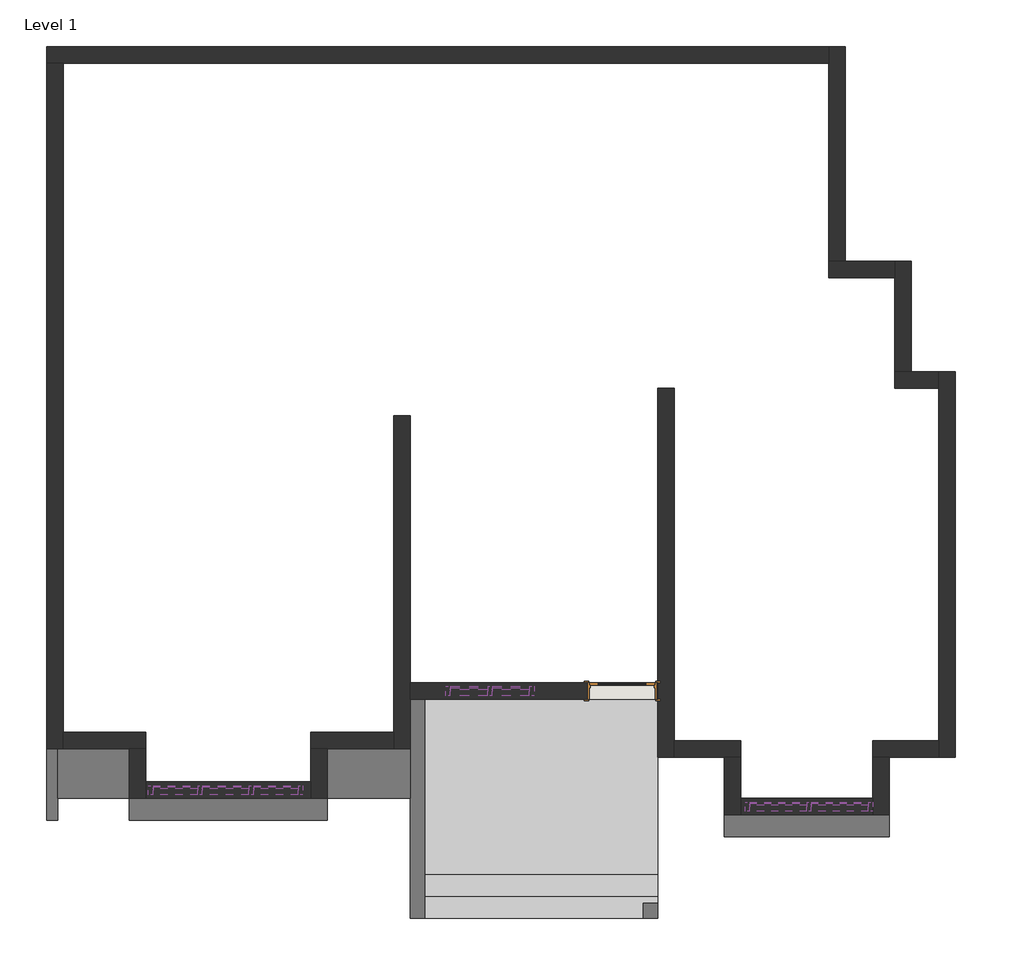
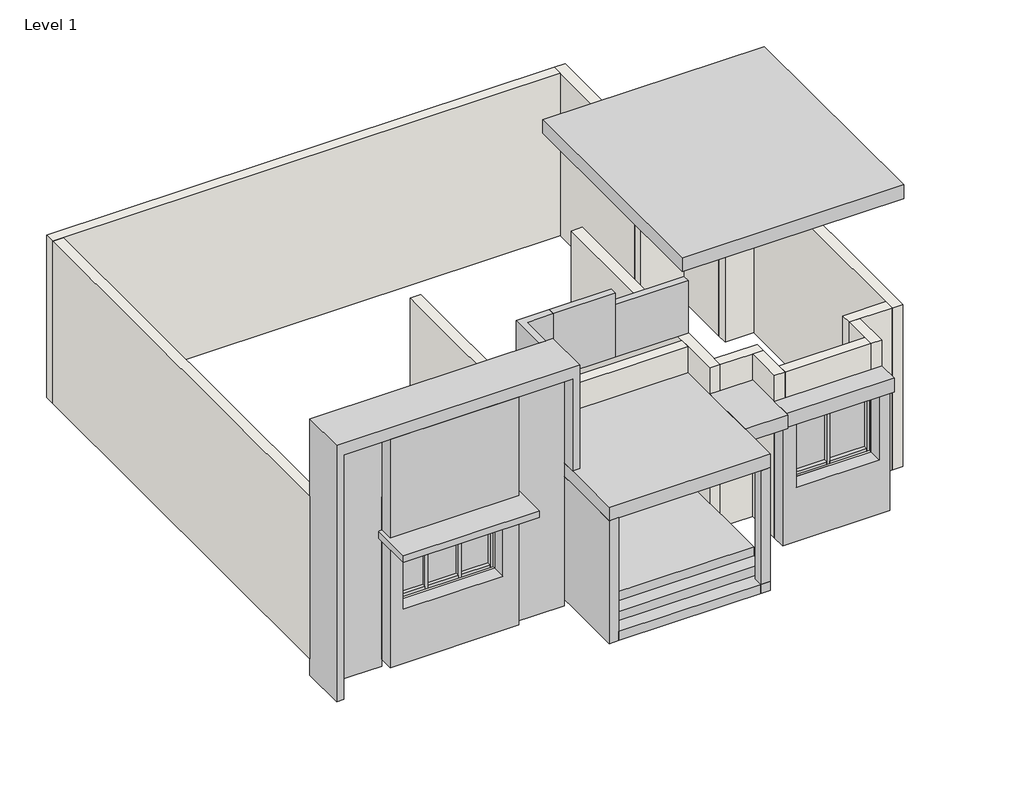
# One storey: 24 members, 20 walls, 7 plates, 1 door, 1 proxy.
"""IFC4 building model written with IfcOpenShell, lengths in millimetres."""

from ifc_helpers import new_model, si_unit, frame, origin, place, context, project, spatial, polyline, outline, extrude, faceted_brep, transform, mapped, element, save
from components import generic_models_1_generic_models_1_0fe661e1, door_3b97b8e7, member_3f0e0172, member_c1df12fd, member_5215b92c, member_fedd83b6, member_0b7646a3, member_429f6687, system_panel_glazed_6c2109f1, system_panel_glazed_f1df731e, system_panel_glazed_57bc90b1, system_panel_glazed_b0c11670

model = new_model("IFC4")

# Units and contexts
model_context = context("Model", 3, world=origin())
ifc_project = project(units=[si_unit("LENGTHUNIT", "METRE", prefix="MILLI")], contexts=[model_context])

# Site, building, storey
site = spatial("IfcSite", under=ifc_project)
building = spatial("IfcBuilding", under=site)
storey = spatial("IfcBuildingStorey", under=building, Name="Level 1", Elevation=0.0)

# Proxy
placement = place(None, origin())
generic_models_1_generic_models_1_shape = generic_models_1_generic_models_1_0fe661e1(model_context)
element("IfcBuildingElementProxy", 1, Name="Generic Models 1 : Generic Models 1", ObjectType="Generic Models 1 : Generic Models 1", at=placement, inside=storey, context=model_context, shape_type="MappedRepresentation", body=[
    mapped(generic_models_1_generic_models_1_shape, transform((0.0, 0.0, 0.0), x_axis=(1.0, 0.0, 0.0), y_axis=(0.0, 1.0, 0.0), z_axis=(0.0, 0.0, 1.0))),
])

# Door
door_shape = door_3b97b8e7(model_context)
element("IfcDoor", 2, ObjectType="Door-Interior-Single-1_Panel-Wood : 3'6\" x 7'", at=placement, inside=storey, context=model_context, shape_type="MappedRepresentation", body=[
    mapped(door_shape, transform((341.9424957, 5044.1158272, 609.6), x_axis=(1.0, 0.0, 0.0), y_axis=(0.0, 1.0, 0.0), z_axis=(0.0, 0.0, 1.0))),
])

# Members
member_shape = member_3f0e0172(model_context)
element("IfcMember", 3, ObjectType="Rectangular Mullion : 2.5\" x 5\" rectangular", at=placement, inside=storey, context=model_context, shape_type="MappedRepresentation", body=[
    mapped(member_shape, transform((-4141.1575043, 3669.3408272, 2768.6), x_axis=(0.0, 0.0, 1.0), y_axis=(0.0, -1.0, 0.0), z_axis=(1.0, 0.0, 0.0))),
])
element("IfcMember", 4, ObjectType="Rectangular Mullion : 2.5\" x 5\" rectangular", at=placement, inside=storey, context=model_context, shape_type="MappedRepresentation", body=[
    mapped(member_shape, transform((-5531.8075043, 3669.3408272, 2768.6), x_axis=(0.0, 0.0, 1.0), y_axis=(0.0, -1.0, 0.0), z_axis=(1.0, 0.0, 0.0))),
])
element("IfcMember", 5, ObjectType="Rectangular Mullion : 2.5\" x 5\" rectangular", at=placement, inside=storey, context=model_context, shape_type="MappedRepresentation", body=[
    mapped(member_shape, transform((-6147.7575043, 3669.3408272, 1219.2), x_axis=(0.0, 0.0, -1.0), y_axis=(0.0, -1.0, 0.0), z_axis=(-1.0, 0.0, 0.0))),
])
element("IfcMember", 6, ObjectType="Rectangular Mullion : 2.5\" x 5\" rectangular", at=placement, inside=storey, context=model_context, shape_type="MappedRepresentation", body=[
    mapped(member_shape, transform((-4757.1075043, 3669.3408272, 1219.2), x_axis=(0.0, 0.0, -1.0), y_axis=(0.0, -1.0, 0.0), z_axis=(-1.0, 0.0, 0.0))),
])
member_2_shape = member_c1df12fd(model_context)
element("IfcMember", 7, ObjectType="Rectangular Mullion : 2.5\" x 5\" rectangular", at=placement, inside=storey, context=model_context, shape_type="MappedRepresentation", body=[
    mapped(member_2_shape, transform((-5500.0575043, 3669.3408272, 1219.2), x_axis=(1.0, 0.0, 0.0), y_axis=(0.0, -1.0, 0.0), z_axis=(0.0, 0.0, -1.0))),
])
element("IfcMember", 8, ObjectType="Rectangular Mullion : 2.5\" x 5\" rectangular", at=placement, inside=storey, context=model_context, shape_type="MappedRepresentation", body=[
    mapped(member_2_shape, transform((-4788.8575043, 3669.3408272, 1219.2), x_axis=(1.0, 0.0, 0.0), y_axis=(0.0, -1.0, 0.0), z_axis=(0.0, 0.0, -1.0))),
])
element("IfcMember", 9, ObjectType="Rectangular Mullion : 2.5\" x 5\" rectangular", at=placement, inside=storey, context=model_context, shape_type="MappedRepresentation", body=[
    mapped(member_2_shape, transform((-1486.8575043, 5040.9408272, 1219.2), x_axis=(1.0, 0.0, 0.0), y_axis=(0.0, -1.0, 0.0), z_axis=(0.0, 0.0, -1.0))),
])
element("IfcMember", 10, ObjectType="Rectangular Mullion : 2.5\" x 5\" rectangular", at=placement, inside=storey, context=model_context, shape_type="MappedRepresentation", body=[
    mapped(member_2_shape, transform((2926.3924957, 3440.7408272, 1219.2), x_axis=(1.0, 0.0, 0.0), y_axis=(0.0, -1.0, 0.0), z_axis=(0.0, 0.0, -1.0))),
])
member_3_shape = member_5215b92c(model_context)
element("IfcMember", 11, ObjectType="Rectangular Mullion : 2.5\" x 5\" rectangular", at=placement, inside=storey, context=model_context, shape_type="MappedRepresentation", body=[
    mapped(member_3_shape, transform((-5468.3075043, 3669.3408272, 1219.2), x_axis=(0.0, 0.0, -1.0), y_axis=(0.0, -1.0, 0.0), z_axis=(-1.0, 0.0, 0.0))),
])
element("IfcMember", 12, ObjectType="Rectangular Mullion : 2.5\" x 5\" rectangular", at=placement, inside=storey, context=model_context, shape_type="MappedRepresentation", body=[
    mapped(member_3_shape, transform((-4820.6075043, 3669.3408272, 2768.6), x_axis=(0.0, 0.0, 1.0), y_axis=(0.0, -1.0, 0.0), z_axis=(1.0, 0.0, 0.0))),
])
member_4_shape = member_fedd83b6(model_context)
element("IfcMember", 13, ObjectType="Rectangular Mullion : 2.5\" x 5\" rectangular", at=placement, inside=storey, context=model_context, shape_type="MappedRepresentation", body=[
    mapped(member_4_shape, transform((-6211.2575043, 3669.3408272, 2768.6), x_axis=(-1.0, 0.0, 0.0), y_axis=(0.0, -1.0, 0.0), z_axis=(0.0, 0.0, 1.0))),
])
element("IfcMember", 14, ObjectType="Rectangular Mullion : 2.5\" x 5\" rectangular", at=placement, inside=storey, context=model_context, shape_type="MappedRepresentation", body=[
    mapped(member_4_shape, transform((-2096.4575043, 5040.9408272, 2768.6), x_axis=(-1.0, 0.0, 0.0), y_axis=(0.0, -1.0, 0.0), z_axis=(0.0, 0.0, 1.0))),
])
element("IfcMember", 15, ObjectType="Rectangular Mullion : 2.5\" x 5\" rectangular", at=placement, inside=storey, context=model_context, shape_type="MappedRepresentation", body=[
    mapped(member_4_shape, transform((2043.7424957, 3440.7408272, 2768.6), x_axis=(-1.0, 0.0, 0.0), y_axis=(0.0, -1.0, 0.0), z_axis=(0.0, 0.0, 1.0))),
])
element("IfcMember", 16, ObjectType="Rectangular Mullion : 2.5\" x 5\" rectangular", at=placement, inside=storey, context=model_context, shape_type="MappedRepresentation", body=[
    mapped(member_4_shape, transform((-4077.6575043, 3669.3408272, 1219.2), x_axis=(1.0, 0.0, 0.0), y_axis=(0.0, -1.0, 0.0), z_axis=(0.0, 0.0, -1.0))),
])
element("IfcMember", 17, ObjectType="Rectangular Mullion : 2.5\" x 5\" rectangular", at=placement, inside=storey, context=model_context, shape_type="MappedRepresentation", body=[
    mapped(member_4_shape, transform((-877.2575043, 5040.9408272, 1219.2), x_axis=(1.0, 0.0, 0.0), y_axis=(0.0, -1.0, 0.0), z_axis=(0.0, 0.0, -1.0))),
])
element("IfcMember", 18, ObjectType="Rectangular Mullion : 2.5\" x 5\" rectangular", at=placement, inside=storey, context=model_context, shape_type="MappedRepresentation", body=[
    mapped(member_4_shape, transform((3809.0424957, 3440.7408272, 1219.2), x_axis=(1.0, 0.0, 0.0), y_axis=(0.0, -1.0, 0.0), z_axis=(0.0, 0.0, -1.0))),
])
member_5_shape = member_0b7646a3(model_context)
element("IfcMember", 19, ObjectType="Rectangular Mullion : 2.5\" x 5\" rectangular", at=placement, inside=storey, context=model_context, shape_type="MappedRepresentation", body=[
    mapped(member_5_shape, transform((-940.7575043, 5040.9408272, 2768.6), x_axis=(0.0, 0.0, 1.0), y_axis=(0.0, -1.0, 0.0), z_axis=(1.0, 0.0, 0.0))),
])
element("IfcMember", 20, ObjectType="Rectangular Mullion : 2.5\" x 5\" rectangular", at=placement, inside=storey, context=model_context, shape_type="MappedRepresentation", body=[
    mapped(member_5_shape, transform((-1518.6075043, 5040.9408272, 2768.6), x_axis=(0.0, 0.0, 1.0), y_axis=(0.0, -1.0, 0.0), z_axis=(1.0, 0.0, 0.0))),
])
element("IfcMember", 21, ObjectType="Rectangular Mullion : 2.5\" x 5\" rectangular", at=placement, inside=storey, context=model_context, shape_type="MappedRepresentation", body=[
    mapped(member_5_shape, transform((-2032.9575043, 5040.9408272, 1219.2), x_axis=(0.0, 0.0, -1.0), y_axis=(0.0, -1.0, 0.0), z_axis=(-1.0, 0.0, 0.0))),
])
element("IfcMember", 22, ObjectType="Rectangular Mullion : 2.5\" x 5\" rectangular", at=placement, inside=storey, context=model_context, shape_type="MappedRepresentation", body=[
    mapped(member_5_shape, transform((-1455.1075043, 5040.9408272, 1219.2), x_axis=(0.0, 0.0, -1.0), y_axis=(0.0, -1.0, 0.0), z_axis=(-1.0, 0.0, 0.0))),
])
member_6_shape = member_429f6687(model_context)
element("IfcMember", 23, ObjectType="Rectangular Mullion : 2.5\" x 5\" rectangular", at=placement, inside=storey, context=model_context, shape_type="MappedRepresentation", body=[
    mapped(member_6_shape, transform((3745.5424957, 3440.7408272, 2768.6), x_axis=(0.0, 0.0, 1.0), y_axis=(0.0, -1.0, 0.0), z_axis=(1.0, 0.0, 0.0))),
])
element("IfcMember", 24, ObjectType="Rectangular Mullion : 2.5\" x 5\" rectangular", at=placement, inside=storey, context=model_context, shape_type="MappedRepresentation", body=[
    mapped(member_6_shape, transform((2894.6424957, 3440.7408272, 2768.6), x_axis=(0.0, 0.0, 1.0), y_axis=(0.0, -1.0, 0.0), z_axis=(1.0, 0.0, 0.0))),
])
element("IfcMember", 25, ObjectType="Rectangular Mullion : 2.5\" x 5\" rectangular", at=placement, inside=storey, context=model_context, shape_type="MappedRepresentation", body=[
    mapped(member_6_shape, transform((2107.2424957, 3440.7408272, 1219.2), x_axis=(0.0, 0.0, -1.0), y_axis=(0.0, -1.0, 0.0), z_axis=(-1.0, 0.0, 0.0))),
])
element("IfcMember", 26, ObjectType="Rectangular Mullion : 2.5\" x 5\" rectangular", at=placement, inside=storey, context=model_context, shape_type="MappedRepresentation", body=[
    mapped(member_6_shape, transform((2958.1424957, 3440.7408272, 1219.2), x_axis=(0.0, 0.0, -1.0), y_axis=(0.0, -1.0, 0.0), z_axis=(-1.0, 0.0, 0.0))),
])

# Plates
system_panel_glazed_shape = system_panel_glazed_6c2109f1(model_context)
element("IfcPlate", 27, ObjectType="System Panel : Glazed", at=placement, inside=storey, context=model_context, shape_type="MappedRepresentation", body=[
    mapped(system_panel_glazed_shape, transform((-5839.7825043, 3669.3408272, 1282.7), x_axis=(1.0, 0.0, 0.0), y_axis=(0.0, 1.0, 0.0), z_axis=(0.0, 0.0, 1.0))),
])
element("IfcPlate", 28, ObjectType="System Panel : Glazed", at=placement, inside=storey, context=model_context, shape_type="MappedRepresentation", body=[
    mapped(system_panel_glazed_shape, transform((-4449.1325043, 3669.3408272, 1282.7), x_axis=(1.0, 0.0, 0.0), y_axis=(0.0, 1.0, 0.0), z_axis=(0.0, 0.0, 1.0))),
])
system_panel_glazed_2_shape = system_panel_glazed_f1df731e(model_context)
element("IfcPlate", 29, ObjectType="System Panel : Glazed", at=placement, inside=storey, context=model_context, shape_type="MappedRepresentation", body=[
    mapped(system_panel_glazed_2_shape, transform((-5144.4575043, 3669.3408272, 1282.7), x_axis=(1.0, 0.0, 0.0), y_axis=(0.0, 1.0, 0.0), z_axis=(0.0, 0.0, 1.0))),
])
system_panel_glazed_3_shape = system_panel_glazed_57bc90b1(model_context)
element("IfcPlate", 30, ObjectType="System Panel : Glazed", at=placement, inside=storey, context=model_context, shape_type="MappedRepresentation", body=[
    mapped(system_panel_glazed_3_shape, transform((-1775.7825043, 5040.9408272, 1282.7), x_axis=(1.0, 0.0, 0.0), y_axis=(0.0, 1.0, 0.0), z_axis=(0.0, 0.0, 1.0))),
])
element("IfcPlate", 31, ObjectType="System Panel : Glazed", at=placement, inside=storey, context=model_context, shape_type="MappedRepresentation", body=[
    mapped(system_panel_glazed_3_shape, transform((-1197.9325043, 5040.9408272, 1282.7), x_axis=(1.0, 0.0, 0.0), y_axis=(0.0, 1.0, 0.0), z_axis=(0.0, 0.0, 1.0))),
])
system_panel_glazed_4_shape = system_panel_glazed_b0c11670(model_context)
element("IfcPlate", 32, ObjectType="System Panel : Glazed", at=placement, inside=storey, context=model_context, shape_type="MappedRepresentation", body=[
    mapped(system_panel_glazed_4_shape, transform((2500.9424957, 3440.7408272, 1282.7), x_axis=(1.0, 0.0, 0.0), y_axis=(0.0, 1.0, 0.0), z_axis=(0.0, 0.0, 1.0))),
])
element("IfcPlate", 33, ObjectType="System Panel : Glazed", at=placement, inside=storey, context=model_context, shape_type="MappedRepresentation", body=[
    mapped(system_panel_glazed_4_shape, transform((3351.8424957, 3440.7408272, 1282.7), x_axis=(1.0, 0.0, 0.0), y_axis=(0.0, 1.0, 0.0), z_axis=(0.0, 0.0, 1.0))),
])

# Walls
element("IfcWall", 34, ObjectType="9\" wall", at=placement, inside=storey, context=model_context, shape_type="Brep", body=[
    faceted_brep([(3199.4424957, 13956.3408272, 0.0), (-7620.9575043, 13956.3408272, 0.0), (-7620.9575043, 13956.3408272, 3657.6), (3199.4424957, 13956.3408272, 3657.6), (3199.4424957, 13727.7408272, 0.0), (3199.4424957, 13727.7408272, 3657.6), (-7392.3575043, 13727.7408272, 3657.6), (-7620.9575043, 13727.7408272, 3657.6), (-7620.9575043, 13727.7408272, 0.0), (-7392.3575043, 13727.7408272, 0.0)], [[[0, 1, 2, 3]], [[4, 5, 6, 7, 8, 9]], [[1, 0, 4, 9, 8]], [[3, 2, 7, 6, 5]], [[2, 1, 8, 7]], [[0, 3, 5, 4]]]),
])
element("IfcWall", 35, ObjectType="9\" wall", at=placement, inside=storey, context=model_context, shape_type="Brep", body=[
    faceted_brep([(-7620.9575043, 13727.7408272, 0.0), (-7620.9575043, 4240.8408272, 0.0), (-7620.9575043, 4240.8408272, 3657.6), (-7620.9575043, 13727.7408272, 3657.6), (-7392.3575043, 13727.7408272, 0.0), (-7392.3575043, 13727.7408272, 3657.6), (-7392.3575043, 4469.4408272, 3657.6), (-7392.3575043, 4240.8408272, 3657.6), (-7392.3575043, 4240.8408272, 0.0), (-7392.3575043, 4469.4408272, 0.0)], [[[0, 1, 2, 3]], [[4, 5, 6, 7, 8, 9]], [[1, 0, 4, 9, 8]], [[3, 2, 7, 6, 5]], [[0, 3, 5, 4]], [[2, 1, 8, 7]]]),
])
element("IfcWall", 36, ObjectType="9\" wall", at=placement, inside=storey, context=model_context, shape_type="Brep", body=[
    faceted_brep([(-2591.7575043, 4240.8408272, 0.0), (-2591.7575043, 4926.6408272, 0.0), (-2591.7575043, 5155.2408272, 0.0), (-2591.7575043, 8850.9408272, 0.0), (-2591.7575043, 8850.9408272, 3657.6), (-2591.7575043, 5155.2408272, 3657.6), (-2591.7575043, 4926.6408272, 3657.6), (-2591.7575043, 4240.8408272, 3657.6), (-2820.3575043, 4240.8408272, 0.0), (-2820.3575043, 4240.8408272, 3657.6), (-2820.3575043, 4469.4408272, 3657.6), (-2820.3575043, 8850.9408272, 3657.6), (-2820.3575043, 8850.9408272, 0.0), (-2820.3575043, 4469.4408272, 0.0)], [[[0, 1, 2, 3, 4, 5, 6, 7]], [[8, 9, 10, 11, 12, 13]], [[3, 2, 1, 0, 8, 13, 12]], [[4, 3, 12, 11]], [[7, 6, 5, 4, 11, 10, 9]], [[0, 7, 9, 8]]]),
])
element("IfcWall", 37, ObjectType="9\" wall", at=placement, inside=storey, context=model_context, shape_type="Brep", body=[
    faceted_brep([(1065.8424957, 4126.5408272, 0.0), (1065.8424957, 4355.1408272, 0.0), (1065.8424957, 9231.9408272, 0.0), (1065.8424957, 9231.9408272, 3657.6), (1065.8424957, 4355.1408272, 3657.6), (1065.8424957, 4126.5408272, 3657.6), (837.2424957, 4126.5408272, 0.0), (837.2424957, 4126.5408272, 3657.6), (837.2424957, 4926.6408272, 3657.6), (837.2424957, 5155.2408272, 3657.6), (837.2424957, 9231.9408272, 3657.6), (837.2424957, 9231.9408272, 0.0), (837.2424957, 5155.2408272, 0.0), (837.2424957, 4926.6408272, 0.0)], [[[0, 1, 2, 3, 4, 5]], [[6, 7, 8, 9, 10, 11, 12, 13]], [[2, 1, 0, 6, 13, 12, 11]], [[3, 2, 11, 10]], [[5, 4, 3, 10, 9, 8, 7]], [[0, 5, 7, 6]]]),
])
element("IfcWall", 38, ObjectType="9\" wall", at=placement, inside=storey, context=model_context, shape_type="Brep", body=[
    faceted_brep([(4952.0424957, 4126.5408272, 0.0), (4952.0424957, 9460.5408272, 0.0), (4952.0424957, 9460.5408272, 3657.6), (4952.0424957, 4126.5408272, 3657.6), (4723.4424957, 4126.5408272, 0.0), (4723.4424957, 4126.5408272, 3657.6), (4723.4424957, 4355.1408272, 3657.6), (4723.4424957, 9231.9408272, 3657.6), (4723.4424957, 9460.5408272, 3657.6), (4723.4424957, 9460.5408272, 0.0), (4723.4424957, 9231.9408272, 0.0), (4723.4424957, 4355.1408272, 0.0)], [[[0, 1, 2, 3]], [[4, 5, 6, 7, 8, 9, 10, 11]], [[1, 0, 4, 11, 10, 9]], [[3, 2, 8, 7, 6, 5]], [[2, 1, 9, 8]], [[0, 3, 5, 4]]]),
])
element("IfcWall", 39, ObjectType="9\" wall", at=placement, inside=storey, context=model_context, shape_type="Brep", body=[
    faceted_brep([(4723.4424957, 9460.5408272, 0.0), (4342.4424957, 9460.5408272, 0.0), (4113.8424957, 9460.5408272, 0.0), (4113.8424957, 9460.5408272, 3657.6), (4342.4424957, 9460.5408272, 3657.6), (4723.4424957, 9460.5408272, 3657.6), (4723.4424957, 9231.9408272, 0.0), (4723.4424957, 9231.9408272, 3657.6), (4113.8424957, 9231.9408272, 3657.6), (4113.8424957, 9231.9408272, 0.0)], [[[0, 1, 2, 3, 4, 5]], [[6, 7, 8, 9]], [[2, 1, 0, 6, 9]], [[5, 4, 3, 8, 7]], [[0, 5, 7, 6]], [[3, 2, 9, 8]]]),
])
element("IfcWall", 40, ObjectType="9\" wall", at=placement, inside=storey, context=model_context, shape_type="Brep", body=[
    faceted_brep([(4342.4424957, 9460.5408272, 0.0), (4342.4424957, 10984.5408272, 0.0), (4342.4424957, 10984.5408272, 3657.6), (4342.4424957, 9460.5408272, 3657.6), (4113.8424957, 9460.5408272, 0.0), (4113.8424957, 9460.5408272, 3657.6), (4113.8424957, 10755.9408272, 3657.6), (4113.8424957, 10984.5408272, 3657.6), (4113.8424957, 10984.5408272, 0.0), (4113.8424957, 10755.9408272, 0.0)], [[[0, 1, 2, 3]], [[4, 5, 6, 7, 8, 9]], [[1, 0, 4, 9, 8]], [[3, 2, 7, 6, 5]], [[0, 3, 5, 4]], [[2, 1, 8, 7]]]),
])
element("IfcWall", 41, ObjectType="9\" wall", at=placement, inside=storey, context=model_context, shape_type="Brep", body=[
    faceted_brep([(4113.8424957, 10984.5408272, 0.0), (3428.0424957, 10984.5408272, 0.0), (3199.4424957, 10984.5408272, 0.0), (3199.4424957, 10984.5408272, 3657.6), (3428.0424957, 10984.5408272, 3657.6), (4113.8424957, 10984.5408272, 3657.6), (4113.8424957, 10755.9408272, 0.0), (4113.8424957, 10755.9408272, 3657.6), (3199.4424957, 10755.9408272, 3657.6), (3199.4424957, 10755.9408272, 0.0)], [[[0, 1, 2, 3, 4, 5]], [[6, 7, 8, 9]], [[2, 1, 0, 6, 9]], [[5, 4, 3, 8, 7]], [[0, 5, 7, 6]], [[3, 2, 9, 8]]]),
])
element("IfcWall", 42, ObjectType="9\" wall", at=placement, inside=storey, context=model_context, shape_type="Brep", body=[
    faceted_brep([(3428.0424957, 10984.5408272, 0.0), (3428.0424957, 13956.3408272, 0.0), (3428.0424957, 13956.3408272, 3657.6), (3428.0424957, 10984.5408272, 3657.6), (3199.4424957, 10984.5408272, 0.0), (3199.4424957, 10984.5408272, 3657.6), (3199.4424957, 13727.7408272, 3657.6), (3199.4424957, 13956.3408272, 3657.6), (3199.4424957, 13956.3408272, 0.0), (3199.4424957, 13727.7408272, 0.0)], [[[0, 1, 2, 3]], [[4, 5, 6, 7, 8, 9]], [[1, 0, 4, 9, 8]], [[3, 2, 7, 6, 5]], [[0, 3, 5, 4]], [[2, 1, 8, 7]]]),
])
element("IfcWall", 43, ObjectType="9\" wall", at=placement, inside=storey, context=model_context, shape_type="SweptSolid", body=[
    extrude(outline(polyline([(0.0, -2591.7575043), (0.0, 837.2424957), (3657.6, 837.2424957), (3657.6, -2591.7575043), (0.0, -2591.7575043)]), holes=[polyline([(2768.6, 824.5424957), (609.6, 824.5424957), (609.6, -140.6575043), (2768.6, -140.6575043), (2768.6, 824.5424957)]), polyline([(1219.2, -2096.4575043), (2768.6, -2096.4575043), (2768.6, -877.2575043), (1219.2, -877.2575043), (1219.2, -2096.4575043)])]), frame((0.0, 4926.6408272, 0.0), z_axis=(0.0, 1.0, 0.0), x_axis=(0.0, 0.0, 1.0)), (0.0, 0.0, 1.0), 228.6),
])
element("IfcWall", 44, ObjectType="9\" wall", at=placement, inside=storey, context=model_context, shape_type="Brep", body=[
    faceted_brep([(-7392.3575043, 4240.8408272, 0.0), (-6477.9575043, 4240.8408272, 0.0), (-6249.3575043, 4240.8408272, 0.0), (-6249.3575043, 4240.8408272, 3657.6), (-6477.9575043, 4240.8408272, 3657.6), (-7392.3575043, 4240.8408272, 3657.6), (-7392.3575043, 4469.4408272, 0.0), (-7392.3575043, 4469.4408272, 3657.6), (-6249.3575043, 4469.4408272, 3657.6), (-6249.3575043, 4469.4408272, 0.0)], [[[0, 1, 2, 3, 4, 5]], [[6, 7, 8, 9]], [[2, 1, 0, 6, 9]], [[5, 4, 3, 8, 7]], [[0, 5, 7, 6]], [[3, 2, 9, 8]]]),
])
element("IfcWall", 45, ObjectType="9\" wall", at=placement, inside=storey, context=model_context, shape_type="Brep", body=[
    faceted_brep([(-6477.9575043, 4240.8408272, 0.0), (-6477.9575043, 3555.0408272, 0.0), (-6477.9575043, 3555.0408272, 3657.6), (-6477.9575043, 4240.8408272, 3657.6), (-6249.3575043, 4240.8408272, 0.0), (-6249.3575043, 4240.8408272, 3657.6), (-6249.3575043, 3783.6408272, 3657.6), (-6249.3575043, 3555.0408272, 3657.6), (-6249.3575043, 3555.0408272, 0.0), (-6249.3575043, 3783.6408272, 0.0)], [[[0, 1, 2, 3]], [[4, 5, 6, 7, 8, 9]], [[1, 0, 4, 9, 8]], [[3, 2, 7, 6, 5]], [[0, 3, 5, 4]], [[2, 1, 8, 7]]]),
])
element("IfcWall", 46, ObjectType="9\" wall", at=placement, inside=storey, context=model_context, shape_type="Brep", body=[
    faceted_brep([(-2820.3575043, 4469.4408272, 0.0), (-3963.3575043, 4469.4408272, 0.0), (-3963.3575043, 4469.4408272, 3657.6), (-2820.3575043, 4469.4408272, 3657.6), (-2820.3575043, 4240.8408272, 0.0), (-2820.3575043, 4240.8408272, 3657.6), (-3734.7575043, 4240.8408272, 3657.6), (-3963.3575043, 4240.8408272, 3657.6), (-3963.3575043, 4240.8408272, 0.0), (-3734.7575043, 4240.8408272, 0.0)], [[[0, 1, 2, 3]], [[4, 5, 6, 7, 8, 9]], [[1, 0, 4, 9, 8]], [[3, 2, 7, 6, 5]], [[0, 3, 5, 4]], [[2, 1, 8, 7]]]),
])
element("IfcWall", 47, ObjectType="9\" wall", at=placement, inside=storey, context=model_context, shape_type="Brep", body=[
    faceted_brep([(-3963.3575043, 4240.8408272, 0.0), (-3963.3575043, 3783.6408272, 0.0), (-3963.3575043, 3555.0408272, 0.0), (-3963.3575043, 3555.0408272, 3657.6), (-3963.3575043, 3783.6408272, 3657.6), (-3963.3575043, 4240.8408272, 3657.6), (-3734.7575043, 4240.8408272, 0.0), (-3734.7575043, 4240.8408272, 3657.6), (-3734.7575043, 3555.0408272, 3657.6), (-3734.7575043, 3555.0408272, 0.0)], [[[0, 1, 2, 3, 4, 5]], [[6, 7, 8, 9]], [[2, 1, 0, 6, 9]], [[5, 4, 3, 8, 7]], [[0, 5, 7, 6]], [[3, 2, 9, 8]]]),
])
element("IfcWall", 48, ObjectType="9\" wall", at=placement, inside=storey, context=model_context, shape_type="Brep", body=[
    faceted_brep([(1065.8424957, 4126.5408272, 0.0), (1751.6424957, 4126.5408272, 0.0), (1980.2424957, 4126.5408272, 0.0), (1980.2424957, 4126.5408272, 3657.6), (1751.6424957, 4126.5408272, 3657.6), (1065.8424957, 4126.5408272, 3657.6), (1065.8424957, 4355.1408272, 0.0), (1065.8424957, 4355.1408272, 3657.6), (1980.2424957, 4355.1408272, 3657.6), (1980.2424957, 4355.1408272, 0.0)], [[[0, 1, 2, 3, 4, 5]], [[6, 7, 8, 9]], [[2, 1, 0, 6, 9]], [[5, 4, 3, 8, 7]], [[0, 5, 7, 6]], [[3, 2, 9, 8]]]),
])
element("IfcWall", 49, ObjectType="9\" wall", at=placement, inside=storey, context=model_context, shape_type="Brep", body=[
    faceted_brep([(1751.6424957, 4126.5408272, 0.0), (1751.6424957, 3326.4408272, 0.0), (1751.6424957, 3326.4408272, 3657.6), (1751.6424957, 4126.5408272, 3657.6), (1980.2424957, 4126.5408272, 0.0), (1980.2424957, 4126.5408272, 3657.6), (1980.2424957, 3555.0408272, 3657.6), (1980.2424957, 3326.4408272, 3657.6), (1980.2424957, 3326.4408272, 0.0), (1980.2424957, 3555.0408272, 0.0)], [[[0, 1, 2, 3]], [[4, 5, 6, 7, 8, 9]], [[1, 0, 4, 9, 8]], [[3, 2, 7, 6, 5]], [[0, 3, 5, 4]], [[2, 1, 8, 7]]]),
])
element("IfcWall", 50, ObjectType="9\" wall", at=placement, inside=storey, context=model_context, shape_type="Brep", body=[
    faceted_brep([(4723.4424957, 4355.1408272, 0.0), (3809.0424957, 4355.1408272, 0.0), (3809.0424957, 4355.1408272, 3657.6), (4723.4424957, 4355.1408272, 3657.6), (4723.4424957, 4126.5408272, 0.0), (4723.4424957, 4126.5408272, 3657.6), (4037.6424957, 4126.5408272, 3657.6), (3809.0424957, 4126.5408272, 3657.6), (3809.0424957, 4126.5408272, 0.0), (4037.6424957, 4126.5408272, 0.0)], [[[0, 1, 2, 3]], [[4, 5, 6, 7, 8, 9]], [[1, 0, 4, 9, 8]], [[3, 2, 7, 6, 5]], [[0, 3, 5, 4]], [[2, 1, 8, 7]]]),
])
element("IfcWall", 51, ObjectType="9\" wall", at=placement, inside=storey, context=model_context, shape_type="Brep", body=[
    faceted_brep([(3809.0424957, 4126.5408272, 0.0), (3809.0424957, 3555.0408272, 0.0), (3809.0424957, 3326.4408272, 0.0), (3809.0424957, 3326.4408272, 3657.6), (3809.0424957, 3555.0408272, 3657.6), (3809.0424957, 4126.5408272, 3657.6), (4037.6424957, 4126.5408272, 0.0), (4037.6424957, 4126.5408272, 3657.6), (4037.6424957, 3326.4408272, 3657.6), (4037.6424957, 3326.4408272, 0.0)], [[[0, 1, 2, 3, 4, 5]], [[6, 7, 8, 9]], [[2, 1, 0, 6, 9]], [[5, 4, 3, 8, 7]], [[0, 5, 7, 6]], [[3, 2, 9, 8]]]),
])
element("IfcWall", 52, ObjectType="9\" wall", at=placement, inside=storey, context=model_context, shape_type="SweptSolid", body=[
    extrude(outline(polyline([(0.0, 1980.2424957), (0.0, 3809.0424957), (1219.2, 3809.0424957), (1219.2, 2043.7424957), (2768.6, 2043.7424957), (2768.6, 3809.0424957), (3657.6, 3809.0424957), (3657.6, 1980.2424957), (0.0, 1980.2424957)])), frame((0.0, 3326.4408272, 0.0), z_axis=(0.0, 1.0, 0.0), x_axis=(0.0, 0.0, 1.0)), (0.0, 0.0, 1.0), 228.6),
])
element("IfcWall", 53, ObjectType="9\" wall", at=placement, inside=storey, context=model_context, shape_type="SweptSolid", body=[
    extrude(outline(polyline([(0.0, -6249.3575043), (0.0, -3963.3575043), (3657.6, -3963.3575043), (3657.6, -6249.3575043), (0.0, -6249.3575043)]), holes=[polyline([(1219.2, -6211.2575043), (2768.6, -6211.2575043), (2768.6, -4077.6575043), (1219.2, -4077.6575043), (1219.2, -6211.2575043)])]), frame((0.0, 3555.0408272, 0.0), z_axis=(0.0, 1.0, 0.0), x_axis=(0.0, 0.0, 1.0)), (0.0, 0.0, 1.0), 228.6),
])

save(model, "model.ifc")

# Revit data of these elements
# Type "Door-Interior-Single-1_Panel-Wood : 3'6\" x 7'"
#   Type Mark = "9"
#   Assembly Code = "C1020300"
#   Analytic Construction = "Wooden"
#   Top Rail = 0' - 4 11/16"
#   Thickness = 0' - 1 3/8"
#   Thermal Resistance (R) = 2.5876 (h·ft²·°F)/BTU
#   Swing Angle [instance default] = 90.00°
#   Stiles = 0' - 4 3/4"
#   Rough Width = 3' - 2"
#   Rough Height = 7' - 1"
#   Height = 7' - 0"
#   Width = 3' - 0"
#   Heat Transfer Coefficient (U) = 0.3865 BTU/(h·ft²·°F)
#   Bottom Rail = 0' - 9 1/8"
#   Trim Material = door
#   Panel Material = door
#   Frame Material = door
#   Door Handle Material = Aluminum
#   Visual Light Transmittance = 0
#   Solar Heat Gain Coefficient = 0
#   Wall Closure = (empty or 0)
#   Function = (empty or 0)
# Type "Rectangular Mullion : 2.5\" x 5\" rectangular"
#   built-in parameter 1007304 = 0.416667 (stored number, unit not read)
#   built-in parameter 1007301 = 0.104167 (stored number, unit not read)
#   built-in parameter 1007300 = 0.104167 (stored number, unit not read)
# Type "System Panel : Glazed"
#   Construction Type Id = "GSP4R"
#   Analytic Construction = "1/8 in Pilkington single glazing"
#   Visual Light Transmittance = 0.9
#   Solar Heat Gain Coefficient = 0.86
#   Heat Transfer Coefficient (U) = 1.18115 BTU/(h·ft²·°F)
#   Define Thermal Properties by = 1
# Type "9\" wall"
#   Assembly Code = "B2010"
#   Layers, outside or top first: 0' - 9" "wall" (function 1)
# Element 1 (IfcBuildingElementProxy, "Generic Models 1 : Generic Models 1")
#   Phase Created = New Construction
#   Materials on its faces: "Gypsum Wall Board", "Grass", "wood"
# Element 2 (IfcDoor, "Door-Interior-Single-1_Panel-Wood : 3'6\" x 7'")
#   Swing Angle = 90.00°
#   Phase Created = New Construction
#   Materials on its faces: "door", "Aluminum"
# Elements 3, 4, 5, 6, 7, 8, 9, 10, 11, 12, 13, 14, 15, 16, 17, 18, 19, 20, 21, 22, 23, 24, 25, 26 (IfcMember, "Rectangular Mullion : 2.5\" x 5\" rectangular")
#   Phase Created = New Construction
# Elements 27, 28, 29, 30, 31, 32, 33 (IfcPlate, "System Panel : Glazed")
#   Phase Created = New Construction
#   Materials on its faces: "Glass"
# Elements 34, 35, 36, 37, 38, 39, 40, 41, 42, 43, 44, 45, 46, 47, 48, 49, 50, 51, 52, 53 (IfcWall, "9\" wall")
#   Top Offset = 0' - 0"
#   Base Offset = 0' - 0"
#   wall height = 12' - 0"
#   Phase Created = New Construction
#   Base Constraint = Level 1
#   Top Constraint = Level 3
#   Materials on its faces: "wall"
# Materials
#   "door": class "Generic", colour RGB 120 120 120, transparency 0, Cost = 0
#   "Aluminum": class "Metal", colour RGB 247 247 247, transparency 0, Description = "Aluminum 6061", Cost = 0
#   "wall": class "Generic", colour RGB 120 120 120, transparency 0, Cost = 0
#   "Gypsum Wall Board": class "Generic", colour RGB 127 127 127, transparency 0, Description = "Gypsum Wall Board", Cost = 0
#   "Grass": class "Generic", colour RGB 104 137 66, transparency 0, Description = "Physical material.", Cost = 0
#   "wood": class "Generic", colour RGB 120 120 120, transparency 0, Cost = 0
#   "Glass": class "Glass", colour RGB 0 128 192, transparency 0.75, Description = "Soda Lime Glass", Cost = 0
